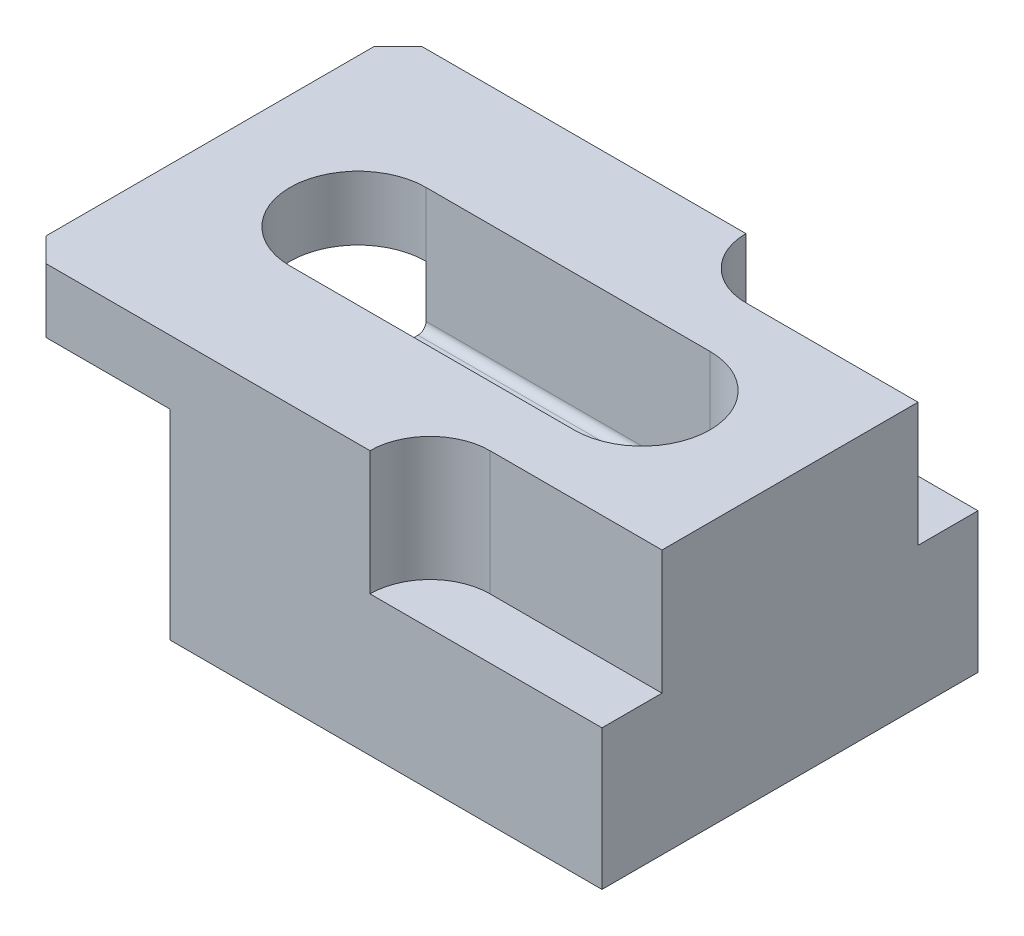
ISO-10303-21;
HEADER;
FILE_DESCRIPTION(('STEP AP214'),'2;1');
FILE_NAME('part.step','',(''),(''),'','','');
FILE_SCHEMA(('AUTOMOTIVE_DESIGN { 1 0 10303 214 1 1 1 1 }'));
ENDSEC;
DATA;
#1=APPLICATION_CONTEXT('core data for automotive mechanical design processes');
#2=APPLICATION_PROTOCOL_DEFINITION('international standard','automotive_design',2000,#1);
#3=PRODUCT_CONTEXT('',#1,'mechanical');
#4=PRODUCT('Part','Part','',(#3));
#5=PRODUCT_RELATED_PRODUCT_CATEGORY('part','',(#4));
#6=PRODUCT_DEFINITION_FORMATION('','',#4);
#7=PRODUCT_DEFINITION_CONTEXT('part definition',#1,'design');
#8=PRODUCT_DEFINITION('design','',#6,#7);
#9=PRODUCT_DEFINITION_SHAPE('','',#8);
#10=(LENGTH_UNIT() NAMED_UNIT(*) SI_UNIT(.MILLI.,.METRE.));
#11=(NAMED_UNIT(*) PLANE_ANGLE_UNIT() SI_UNIT($,.RADIAN.));
#12=(NAMED_UNIT(*) SI_UNIT($,.STERADIAN.) SOLID_ANGLE_UNIT());
#13=UNCERTAINTY_MEASURE_WITH_UNIT(LENGTH_MEASURE(1.E-05),#10,'distance_accuracy_value','');
#14=(GEOMETRIC_REPRESENTATION_CONTEXT(3) GLOBAL_UNCERTAINTY_ASSIGNED_CONTEXT((#13)) GLOBAL_UNIT_ASSIGNED_CONTEXT((#10,
#11,#12)) REPRESENTATION_CONTEXT('',''));
#15=CARTESIAN_POINT('',(0.,0.,0.));
#16=DIRECTION('',(0.,0.,1.));
#17=DIRECTION('',(1.,0.,0.));
#18=AXIS2_PLACEMENT_3D('',#15,#16,#17);
#19=CARTESIAN_POINT('',(-17.75,0.,-8.5));
#20=DIRECTION('',(0.,0.,-1.));
#21=DIRECTION('',(-1.,0.,0.));
#22=AXIS2_PLACEMENT_3D('',#19,#20,#21);
#23=PLANE('',#22);
#24=DIRECTION('',(0.,1.,0.));
#25=VECTOR('',#24,1.);
#26=CARTESIAN_POINT('',(-17.7499999999999,-25.,-8.5));
#27=LINE('',#26,#25);
#28=CARTESIAN_POINT('',(-17.7499999999999,-6.5,-8.5));
#29=VERTEX_POINT('',#28);
#30=CARTESIAN_POINT('',(-17.7499999999999,0.,-8.5));
#31=VERTEX_POINT('',#30);
#32=EDGE_CURVE('E261',#29,#31,#27,.T.);
#33=ORIENTED_EDGE('',*,*,#32,.F.);
#34=DIRECTION('',(-1.,0.,0.));
#35=VECTOR('',#34,1.);
#36=CARTESIAN_POINT('',(17.75,-6.5,-8.5));
#37=LINE('',#36,#35);
#38=CARTESIAN_POINT('',(17.75,-6.5,-8.5));
#39=VERTEX_POINT('',#38);
#40=EDGE_CURVE('E68',#29,#39,#37,.F.);
#41=ORIENTED_EDGE('',*,*,#40,.T.);
#42=DIRECTION('',(0.,1.,0.));
#43=VECTOR('',#42,1.);
#44=CARTESIAN_POINT('',(17.75,0.,-8.5));
#45=LINE('',#44,#43);
#46=CARTESIAN_POINT('',(17.75,8.,-8.5));
#47=VERTEX_POINT('',#46);
#48=EDGE_CURVE('E289',#39,#47,#45,.T.);
#49=ORIENTED_EDGE('',*,*,#48,.T.);
#50=DIRECTION('',(-1.,0.,0.));
#51=VECTOR('',#50,1.);
#52=CARTESIAN_POINT('',(-17.75,8.,-8.5));
#53=LINE('',#52,#51);
#54=CARTESIAN_POINT('',(-17.75,8.,-8.5));
#55=VERTEX_POINT('',#54);
#56=EDGE_CURVE('E273',#47,#55,#53,.T.);
#57=ORIENTED_EDGE('',*,*,#56,.T.);
#58=DIRECTION('',(0.,1.,0.));
#59=VECTOR('',#58,1.);
#60=CARTESIAN_POINT('',(-17.75,0.,-8.5));
#61=LINE('',#60,#59);
#62=EDGE_CURVE('E282',#31,#55,#61,.T.);
#63=ORIENTED_EDGE('',*,*,#62,.F.);
#64=EDGE_LOOP('',(#33,#41,#49,#57,#63));
#65=FACE_BOUND('',#64,.T.);
#66=ADVANCED_FACE('F50',(#65),#23,.F.);
#67=CARTESIAN_POINT('',(17.75,0.,0.));
#68=DIRECTION('',(0.,1.,0.));
#69=DIRECTION('',(0.,0.,1.));
#70=AXIS2_PLACEMENT_3D('',#67,#68,#69);
#71=CYLINDRICAL_SURFACE('',#70,8.5);
#72=ORIENTED_EDGE('',*,*,#48,.F.);
#73=CARTESIAN_POINT('',(17.75,-6.5,0.));
#74=DIRECTION('',(0.,-1.,0.));
#75=DIRECTION('',(0.,0.,-1.));
#76=AXIS2_PLACEMENT_3D('',#73,#74,#75);
#77=CIRCLE('',#76,8.5);
#78=CARTESIAN_POINT('',(17.75,-6.5,8.5));
#79=VERTEX_POINT('',#78);
#80=EDGE_CURVE('E353',#39,#79,#77,.T.);
#81=ORIENTED_EDGE('',*,*,#80,.T.);
#82=DIRECTION('',(0.,1.,0.));
#83=VECTOR('',#82,1.);
#84=CARTESIAN_POINT('',(17.75,0.,8.5));
#85=LINE('',#84,#83);
#86=CARTESIAN_POINT('',(17.75,8.,8.5));
#87=VERTEX_POINT('',#86);
#88=EDGE_CURVE('E290',#79,#87,#85,.T.);
#89=ORIENTED_EDGE('',*,*,#88,.T.);
#90=CARTESIAN_POINT('',(17.75,8.,0.));
#91=DIRECTION('',(0.,1.,0.));
#92=DIRECTION('',(0.,0.,1.));
#93=AXIS2_PLACEMENT_3D('',#90,#91,#92);
#94=CIRCLE('',#93,8.5);
#95=EDGE_CURVE('E278',#87,#47,#94,.T.);
#96=ORIENTED_EDGE('',*,*,#95,.T.);
#97=EDGE_LOOP('',(#72,#81,#89,#96));
#98=FACE_BOUND('',#97,.T.);
#99=ADVANCED_FACE('F388',(#98),#71,.F.);
#100=CARTESIAN_POINT('',(-17.75,0.,8.5));
#101=DIRECTION('',(0.,0.,1.));
#102=DIRECTION('',(1.,0.,0.));
#103=AXIS2_PLACEMENT_3D('',#100,#101,#102);
#104=PLANE('',#103);
#105=ORIENTED_EDGE('',*,*,#88,.F.);
#106=DIRECTION('',(1.,0.,0.));
#107=VECTOR('',#106,1.);
#108=CARTESIAN_POINT('',(-17.75,-6.5,8.5));
#109=LINE('',#108,#107);
#110=CARTESIAN_POINT('',(-17.7499999999999,-6.5,8.5));
#111=VERTEX_POINT('',#110);
#112=EDGE_CURVE('E352',#79,#111,#109,.F.);
#113=ORIENTED_EDGE('',*,*,#112,.T.);
#114=DIRECTION('',(0.,1.,0.));
#115=VECTOR('',#114,1.);
#116=CARTESIAN_POINT('',(-17.7499999999999,-25.,8.5));
#117=LINE('',#116,#115);
#118=CARTESIAN_POINT('',(-17.7499999999999,0.,8.5));
#119=VERTEX_POINT('',#118);
#120=EDGE_CURVE('E258',#111,#119,#117,.T.);
#121=ORIENTED_EDGE('',*,*,#120,.T.);
#122=DIRECTION('',(0.,1.,0.));
#123=VECTOR('',#122,1.);
#124=CARTESIAN_POINT('',(-17.75,0.,8.5));
#125=LINE('',#124,#123);
#126=CARTESIAN_POINT('',(-17.75,8.,8.5));
#127=VERTEX_POINT('',#126);
#128=EDGE_CURVE('E274',#119,#127,#125,.T.);
#129=ORIENTED_EDGE('',*,*,#128,.T.);
#130=DIRECTION('',(1.,0.,0.));
#131=VECTOR('',#130,1.);
#132=CARTESIAN_POINT('',(-17.75,8.,8.5));
#133=LINE('',#132,#131);
#134=EDGE_CURVE('E280',#127,#87,#133,.T.);
#135=ORIENTED_EDGE('',*,*,#134,.T.);
#136=EDGE_LOOP('',(#105,#113,#121,#129,#135));
#137=FACE_BOUND('',#136,.T.);
#138=ADVANCED_FACE('F387',(#137),#104,.F.);
#139=CARTESIAN_POINT('',(7.24999999999998,-17.,16.));
#140=DIRECTION('',(0.,0.,-1.));
#141=DIRECTION('',(-1.,0.,0.));
#142=AXIS2_PLACEMENT_3D('',#139,#140,#141);
#143=PLANE('',#142);
#144=DIRECTION('',(-1.,0.,0.));
#145=VECTOR('',#144,1.);
#146=CARTESIAN_POINT('',(7.24999999999998,-7.5,16.));
#147=LINE('',#146,#145);
#148=CARTESIAN_POINT('',(36.25,-7.5,16.));
#149=VERTEX_POINT('',#148);
#150=CARTESIAN_POINT('',(14.75,-7.5,16.));
#151=VERTEX_POINT('',#150);
#152=EDGE_CURVE('E227',#149,#151,#147,.T.);
#153=ORIENTED_EDGE('',*,*,#152,.F.);
#154=DIRECTION('',(0.,1.,0.));
#155=VECTOR('',#154,1.);
#156=CARTESIAN_POINT('',(36.25,-17.,16.));
#157=LINE('',#156,#155);
#158=CARTESIAN_POINT('',(36.25,8.,16.));
#159=VERTEX_POINT('',#158);
#160=EDGE_CURVE('E237',#149,#159,#157,.T.);
#161=ORIENTED_EDGE('',*,*,#160,.T.);
#162=DIRECTION('',(-1.,0.,0.));
#163=VECTOR('',#162,1.);
#164=CARTESIAN_POINT('',(7.24999999999998,8.,16.));
#165=LINE('',#164,#163);
#166=CARTESIAN_POINT('',(14.75,8.,16.));
#167=VERTEX_POINT('',#166);
#168=EDGE_CURVE('E232',#159,#167,#165,.T.);
#169=ORIENTED_EDGE('',*,*,#168,.T.);
#170=DIRECTION('',(0.,1.,0.));
#171=VECTOR('',#170,1.);
#172=CARTESIAN_POINT('',(14.75,-17.,16.));
#173=LINE('',#172,#171);
#174=EDGE_CURVE('E333',#167,#151,#173,.F.);
#175=ORIENTED_EDGE('',*,*,#174,.T.);
#176=EDGE_LOOP('',(#153,#161,#169,#175));
#177=FACE_BOUND('',#176,.T.);
#178=ADVANCED_FACE('F408',(#177),#143,.F.);
#179=CARTESIAN_POINT('',(36.25,-17.,-16.));
#180=DIRECTION('',(0.,0.,1.));
#181=DIRECTION('',(1.,0.,0.));
#182=AXIS2_PLACEMENT_3D('',#179,#180,#181);
#183=PLANE('',#182);
#184=DIRECTION('',(1.,0.,0.));
#185=VECTOR('',#184,1.);
#186=CARTESIAN_POINT('',(36.25,-7.5,-16.));
#187=LINE('',#186,#185);
#188=CARTESIAN_POINT('',(14.75,-7.5,-16.));
#189=VERTEX_POINT('',#188);
#190=CARTESIAN_POINT('',(36.25,-7.5,-16.));
#191=VERTEX_POINT('',#190);
#192=EDGE_CURVE('E208',#189,#191,#187,.T.);
#193=ORIENTED_EDGE('',*,*,#192,.F.);
#194=DIRECTION('',(0.,1.,0.));
#195=VECTOR('',#194,1.);
#196=CARTESIAN_POINT('',(14.75,8.,-16.));
#197=LINE('',#196,#195);
#198=CARTESIAN_POINT('',(14.75,8.,-16.));
#199=VERTEX_POINT('',#198);
#200=EDGE_CURVE('E332',#189,#199,#197,.T.);
#201=ORIENTED_EDGE('',*,*,#200,.T.);
#202=DIRECTION('',(1.,0.,0.));
#203=VECTOR('',#202,1.);
#204=CARTESIAN_POINT('',(36.25,8.,-16.));
#205=LINE('',#204,#203);
#206=CARTESIAN_POINT('',(36.25,8.,-16.));
#207=VERTEX_POINT('',#206);
#208=EDGE_CURVE('E236',#199,#207,#205,.T.);
#209=ORIENTED_EDGE('',*,*,#208,.T.);
#210=DIRECTION('',(0.,1.,0.));
#211=VECTOR('',#210,1.);
#212=CARTESIAN_POINT('',(36.25,-17.,-16.));
#213=LINE('',#212,#211);
#214=EDGE_CURVE('E239',#191,#207,#213,.T.);
#215=ORIENTED_EDGE('',*,*,#214,.F.);
#216=EDGE_LOOP('',(#193,#201,#209,#215));
#217=FACE_BOUND('',#216,.T.);
#218=ADVANCED_FACE('F454',(#217),#183,.F.);
#219=CARTESIAN_POINT('',(14.75,-17.,-23.5));
#220=DIRECTION('',(0.,-1.,0.));
#221=DIRECTION('',(0.,0.,-1.));
#222=AXIS2_PLACEMENT_3D('',#219,#220,#221);
#223=CYLINDRICAL_SURFACE('',#222,7.5);
#224=CARTESIAN_POINT('',(14.75,-7.5,-23.5));
#225=DIRECTION('',(0.,-1.,0.));
#226=DIRECTION('',(0.,0.,-1.));
#227=AXIS2_PLACEMENT_3D('',#224,#225,#226);
#228=CIRCLE('',#227,7.5);
#229=CARTESIAN_POINT('',(7.24999999999998,-7.5,-23.5));
#230=VERTEX_POINT('',#229);
#231=EDGE_CURVE('E230',#230,#189,#228,.F.);
#232=ORIENTED_EDGE('',*,*,#231,.F.);
#233=DIRECTION('',(0.,1.,0.));
#234=VECTOR('',#233,1.);
#235=CARTESIAN_POINT('',(7.24999999999998,-17.,-23.5));
#236=LINE('',#235,#234);
#237=CARTESIAN_POINT('',(7.24999999999998,8.,-23.5));
#238=VERTEX_POINT('',#237);
#239=EDGE_CURVE('E219',#230,#238,#236,.T.);
#240=ORIENTED_EDGE('',*,*,#239,.T.);
#241=CARTESIAN_POINT('',(14.75,8.,-23.5));
#242=DIRECTION('',(0.,1.,0.));
#243=DIRECTION('',(0.,0.,1.));
#244=AXIS2_PLACEMENT_3D('',#241,#242,#243);
#245=CIRCLE('',#244,7.5);
#246=EDGE_CURVE('E340',#199,#238,#245,.F.);
#247=ORIENTED_EDGE('',*,*,#246,.F.);
#248=ORIENTED_EDGE('',*,*,#200,.F.);
#249=EDGE_LOOP('',(#232,#240,#247,#248));
#250=FACE_BOUND('',#249,.T.);
#251=ADVANCED_FACE('F448',(#250),#223,.F.);
#252=CARTESIAN_POINT('',(14.75,-17.,23.5));
#253=DIRECTION('',(0.,-1.,0.));
#254=DIRECTION('',(0.,0.,-1.));
#255=AXIS2_PLACEMENT_3D('',#252,#253,#254);
#256=CYLINDRICAL_SURFACE('',#255,7.5);
#257=CARTESIAN_POINT('',(14.75,-7.5,23.5));
#258=DIRECTION('',(0.,-1.,0.));
#259=DIRECTION('',(0.,0.,-1.));
#260=AXIS2_PLACEMENT_3D('',#257,#258,#259);
#261=CIRCLE('',#260,7.5);
#262=CARTESIAN_POINT('',(7.24999999999998,-7.5,23.5));
#263=VERTEX_POINT('',#262);
#264=EDGE_CURVE('E345',#151,#263,#261,.F.);
#265=ORIENTED_EDGE('',*,*,#264,.F.);
#266=ORIENTED_EDGE('',*,*,#174,.F.);
#267=CARTESIAN_POINT('',(14.75,8.,23.5));
#268=DIRECTION('',(0.,1.,0.));
#269=DIRECTION('',(0.,0.,1.));
#270=AXIS2_PLACEMENT_3D('',#267,#268,#269);
#271=CIRCLE('',#270,7.5);
#272=CARTESIAN_POINT('',(7.24999999999998,8.,23.5));
#273=VERTEX_POINT('',#272);
#274=EDGE_CURVE('E338',#273,#167,#271,.F.);
#275=ORIENTED_EDGE('',*,*,#274,.F.);
#276=DIRECTION('',(0.,1.,0.));
#277=VECTOR('',#276,1.);
#278=CARTESIAN_POINT('',(7.24999999999998,-17.,23.5));
#279=LINE('',#278,#277);
#280=EDGE_CURVE('E244',#263,#273,#279,.T.);
#281=ORIENTED_EDGE('',*,*,#280,.F.);
#282=EDGE_LOOP('',(#265,#266,#275,#281));
#283=FACE_BOUND('',#282,.T.);
#284=ADVANCED_FACE('F436',(#283),#256,.F.);
#285=CARTESIAN_POINT('',(36.25,8.,-23.5));
#286=DIRECTION('',(-1.,0.,0.));
#287=DIRECTION('',(0.,0.,1.));
#288=AXIS2_PLACEMENT_3D('',#285,#286,#287);
#289=PLANE('',#288);
#290=DIRECTION('',(0.,0.,-1.));
#291=VECTOR('',#290,1.);
#292=CARTESIAN_POINT('',(36.25,-7.5,-23.5));
#293=LINE('',#292,#291);
#294=CARTESIAN_POINT('',(36.25,-7.5,-23.5));
#295=VERTEX_POINT('',#294);
#296=EDGE_CURVE('E191',#191,#295,#293,.T.);
#297=ORIENTED_EDGE('',*,*,#296,.F.);
#298=ORIENTED_EDGE('',*,*,#214,.T.);
#299=DIRECTION('',(0.,0.,-1.));
#300=VECTOR('',#299,1.);
#301=CARTESIAN_POINT('',(36.25,8.,-23.5));
#302=LINE('',#301,#300);
#303=EDGE_CURVE('E295',#159,#207,#302,.T.);
#304=ORIENTED_EDGE('',*,*,#303,.F.);
#305=ORIENTED_EDGE('',*,*,#160,.F.);
#306=CARTESIAN_POINT('',(36.25,-7.5,23.5));
#307=VERTEX_POINT('',#306);
#308=EDGE_CURVE('E212',#307,#149,#293,.T.);
#309=ORIENTED_EDGE('',*,*,#308,.F.);
#310=DIRECTION('',(0.,-1.,0.));
#311=VECTOR('',#310,1.);
#312=CARTESIAN_POINT('',(36.25,8.,23.5));
#313=LINE('',#312,#311);
#314=CARTESIAN_POINT('',(36.25,-25.,23.5));
#315=VERTEX_POINT('',#314);
#316=EDGE_CURVE('E202',#307,#315,#313,.T.);
#317=ORIENTED_EDGE('',*,*,#316,.T.);
#318=DIRECTION('',(0.,0.,-1.));
#319=VECTOR('',#318,1.);
#320=CARTESIAN_POINT('',(36.25,-25.,-23.5));
#321=LINE('',#320,#319);
#322=CARTESIAN_POINT('',(36.25,-25.,-23.5));
#323=VERTEX_POINT('',#322);
#324=EDGE_CURVE('E199',#315,#323,#321,.T.);
#325=ORIENTED_EDGE('',*,*,#324,.T.);
#326=DIRECTION('',(0.,-1.,0.));
#327=VECTOR('',#326,1.);
#328=CARTESIAN_POINT('',(36.25,8.,-23.5));
#329=LINE('',#328,#327);
#330=EDGE_CURVE('E192',#295,#323,#329,.T.);
#331=ORIENTED_EDGE('',*,*,#330,.F.);
#332=EDGE_LOOP('',(#297,#298,#304,#305,#309,#317,#325,#331));
#333=FACE_BOUND('',#332,.T.);
#334=ADVANCED_FACE('F194',(#333),#289,.F.);
#335=CARTESIAN_POINT('',(-36.25,8.,-23.5));
#336=DIRECTION('',(0.,0.,1.));
#337=DIRECTION('',(1.,0.,0.));
#338=AXIS2_PLACEMENT_3D('',#335,#336,#337);
#339=PLANE('',#338);
#340=DIRECTION('',(0.,1.,0.));
#341=VECTOR('',#340,1.);
#342=CARTESIAN_POINT('',(-17.7499999999999,-25.,-23.5));
#343=LINE('',#342,#341);
#344=CARTESIAN_POINT('',(-17.7499999999999,-25.,-23.5));
#345=VERTEX_POINT('',#344);
#346=CARTESIAN_POINT('',(-17.7499999999999,0.,-23.5));
#347=VERTEX_POINT('',#346);
#348=EDGE_CURVE('E257',#345,#347,#343,.T.);
#349=ORIENTED_EDGE('',*,*,#348,.T.);
#350=DIRECTION('',(-1.,0.,0.));
#351=VECTOR('',#350,1.);
#352=CARTESIAN_POINT('',(-36.25,0.,-23.5));
#353=LINE('',#352,#351);
#354=CARTESIAN_POINT('',(-33.25,0.,-23.5));
#355=VERTEX_POINT('',#354);
#356=EDGE_CURVE('E287',#347,#355,#353,.T.);
#357=ORIENTED_EDGE('',*,*,#356,.T.);
#358=DIRECTION('',(0.,1.,0.));
#359=VECTOR('',#358,1.);
#360=CARTESIAN_POINT('',(-33.25,8.,-23.5));
#361=LINE('',#360,#359);
#362=CARTESIAN_POINT('',(-33.25,8.,-23.5));
#363=VERTEX_POINT('',#362);
#364=EDGE_CURVE('E325',#355,#363,#361,.T.);
#365=ORIENTED_EDGE('',*,*,#364,.T.);
#366=DIRECTION('',(-1.,0.,0.));
#367=VECTOR('',#366,1.);
#368=CARTESIAN_POINT('',(-36.25,8.,-23.5));
#369=LINE('',#368,#367);
#370=EDGE_CURVE('E300',#238,#363,#369,.T.);
#371=ORIENTED_EDGE('',*,*,#370,.F.);
#372=ORIENTED_EDGE('',*,*,#239,.F.);
#373=DIRECTION('',(-1.,0.,0.));
#374=VECTOR('',#373,1.);
#375=CARTESIAN_POINT('',(36.25,-7.5,-23.5));
#376=LINE('',#375,#374);
#377=EDGE_CURVE('E209',#295,#230,#376,.T.);
#378=ORIENTED_EDGE('',*,*,#377,.F.);
#379=ORIENTED_EDGE('',*,*,#330,.T.);
#380=DIRECTION('',(-1.,0.,0.));
#381=VECTOR('',#380,1.);
#382=CARTESIAN_POINT('',(36.25,-25.,-23.5));
#383=LINE('',#382,#381);
#384=EDGE_CURVE('E248',#323,#345,#383,.T.);
#385=ORIENTED_EDGE('',*,*,#384,.T.);
#386=EDGE_LOOP('',(#349,#357,#365,#371,#372,#378,#379,#385));
#387=FACE_BOUND('',#386,.T.);
#388=ADVANCED_FACE('F211',(#387),#339,.F.);
#389=CARTESIAN_POINT('',(-36.25,8.,-23.5));
#390=DIRECTION('',(1.,0.,0.));
#391=DIRECTION('',(0.,0.,-1.));
#392=AXIS2_PLACEMENT_3D('',#389,#390,#391);
#393=PLANE('',#392);
#394=DIRECTION('',(0.,0.,1.));
#395=VECTOR('',#394,1.);
#396=CARTESIAN_POINT('',(-36.25,8.,-23.5));
#397=LINE('',#396,#395);
#398=CARTESIAN_POINT('',(-36.25,8.,-20.5));
#399=VERTEX_POINT('',#398);
#400=CARTESIAN_POINT('',(-36.25,8.,20.5));
#401=VERTEX_POINT('',#400);
#402=EDGE_CURVE('E297',#399,#401,#397,.T.);
#403=ORIENTED_EDGE('',*,*,#402,.F.);
#404=DIRECTION('',(0.,-1.,0.));
#405=VECTOR('',#404,1.);
#406=CARTESIAN_POINT('',(-36.25,8.,-20.5));
#407=LINE('',#406,#405);
#408=CARTESIAN_POINT('',(-36.25,0.,-20.5));
#409=VERTEX_POINT('',#408);
#410=EDGE_CURVE('E313',#399,#409,#407,.T.);
#411=ORIENTED_EDGE('',*,*,#410,.T.);
#412=DIRECTION('',(0.,0.,1.));
#413=VECTOR('',#412,1.);
#414=CARTESIAN_POINT('',(-36.25,0.,-23.5));
#415=LINE('',#414,#413);
#416=CARTESIAN_POINT('',(-36.25,0.,20.5));
#417=VERTEX_POINT('',#416);
#418=EDGE_CURVE('E310',#409,#417,#415,.T.);
#419=ORIENTED_EDGE('',*,*,#418,.T.);
#420=DIRECTION('',(0.,1.,0.));
#421=VECTOR('',#420,1.);
#422=CARTESIAN_POINT('',(-36.25,8.,20.5));
#423=LINE('',#422,#421);
#424=EDGE_CURVE('E201',#417,#401,#423,.T.);
#425=ORIENTED_EDGE('',*,*,#424,.T.);
#426=EDGE_LOOP('',(#403,#411,#419,#425));
#427=FACE_BOUND('',#426,.T.);
#428=ADVANCED_FACE('F430',(#427),#393,.F.);
#429=CARTESIAN_POINT('',(-36.25,8.,23.5));
#430=DIRECTION('',(0.,0.,-1.));
#431=DIRECTION('',(-1.,0.,0.));
#432=AXIS2_PLACEMENT_3D('',#429,#430,#431);
#433=PLANE('',#432);
#434=DIRECTION('',(1.,0.,0.));
#435=VECTOR('',#434,1.);
#436=CARTESIAN_POINT('',(-36.25,0.,23.5));
#437=LINE('',#436,#435);
#438=CARTESIAN_POINT('',(-33.25,0.,23.5));
#439=VERTEX_POINT('',#438);
#440=CARTESIAN_POINT('',(-17.7499999999999,0.,23.5));
#441=VERTEX_POINT('',#440);
#442=EDGE_CURVE('E296',#439,#441,#437,.T.);
#443=ORIENTED_EDGE('',*,*,#442,.T.);
#444=DIRECTION('',(0.,1.,0.));
#445=VECTOR('',#444,1.);
#446=CARTESIAN_POINT('',(-17.7499999999999,-25.,23.5));
#447=LINE('',#446,#445);
#448=CARTESIAN_POINT('',(-17.7499999999999,-25.,23.5));
#449=VERTEX_POINT('',#448);
#450=EDGE_CURVE('E260',#449,#441,#447,.T.);
#451=ORIENTED_EDGE('',*,*,#450,.F.);
#452=DIRECTION('',(1.,0.,0.));
#453=VECTOR('',#452,1.);
#454=CARTESIAN_POINT('',(36.25,-25.,23.5));
#455=LINE('',#454,#453);
#456=EDGE_CURVE('E254',#449,#315,#455,.T.);
#457=ORIENTED_EDGE('',*,*,#456,.T.);
#458=ORIENTED_EDGE('',*,*,#316,.F.);
#459=DIRECTION('',(1.,0.,0.));
#460=VECTOR('',#459,1.);
#461=CARTESIAN_POINT('',(36.25,-7.5,23.5));
#462=LINE('',#461,#460);
#463=EDGE_CURVE('E221',#263,#307,#462,.T.);
#464=ORIENTED_EDGE('',*,*,#463,.F.);
#465=ORIENTED_EDGE('',*,*,#280,.T.);
#466=DIRECTION('',(1.,0.,0.));
#467=VECTOR('',#466,1.);
#468=CARTESIAN_POINT('',(-36.25,8.,23.5));
#469=LINE('',#468,#467);
#470=CARTESIAN_POINT('',(-33.25,8.,23.5));
#471=VERTEX_POINT('',#470);
#472=EDGE_CURVE('E303',#471,#273,#469,.T.);
#473=ORIENTED_EDGE('',*,*,#472,.F.);
#474=DIRECTION('',(0.,-1.,0.));
#475=VECTOR('',#474,1.);
#476=CARTESIAN_POINT('',(-33.25,8.,23.5));
#477=LINE('',#476,#475);
#478=EDGE_CURVE('E328',#471,#439,#477,.T.);
#479=ORIENTED_EDGE('',*,*,#478,.T.);
#480=EDGE_LOOP('',(#443,#451,#457,#458,#464,#465,#473,#479));
#481=FACE_BOUND('',#480,.T.);
#482=ADVANCED_FACE('F420',(#481),#433,.F.);
#483=CARTESIAN_POINT('',(0.,8.,0.));
#484=DIRECTION('',(0.,1.,0.));
#485=DIRECTION('',(0.,0.,1.));
#486=AXIS2_PLACEMENT_3D('',#483,#484,#485);
#487=PLANE('',#486);
#488=ORIENTED_EDGE('',*,*,#208,.F.);
#489=ORIENTED_EDGE('',*,*,#246,.T.);
#490=ORIENTED_EDGE('',*,*,#370,.T.);
#491=DIRECTION('',(0.707106781186548,0.,-0.707106781186547));
#492=VECTOR('',#491,1.);
#493=CARTESIAN_POINT('',(-28.375,8.,-28.375));
#494=LINE('',#493,#492);
#495=EDGE_CURVE('E326',#363,#399,#494,.F.);
#496=ORIENTED_EDGE('',*,*,#495,.T.);
#497=ORIENTED_EDGE('',*,*,#402,.T.);
#498=DIRECTION('',(-0.707106781186547,0.,-0.707106781186548));
#499=VECTOR('',#498,1.);
#500=CARTESIAN_POINT('',(-28.375,8.,28.375));
#501=LINE('',#500,#499);
#502=EDGE_CURVE('E323',#401,#471,#501,.F.);
#503=ORIENTED_EDGE('',*,*,#502,.T.);
#504=ORIENTED_EDGE('',*,*,#472,.T.);
#505=ORIENTED_EDGE('',*,*,#274,.T.);
#506=ORIENTED_EDGE('',*,*,#168,.F.);
#507=ORIENTED_EDGE('',*,*,#303,.T.);
#508=EDGE_LOOP('',(#488,#489,#490,#496,#497,#503,#504,#505,#506,#507));
#509=FACE_BOUND('',#508,.T.);
#510=ORIENTED_EDGE('',*,*,#134,.F.);
#511=CARTESIAN_POINT('',(-17.75,8.,0.));
#512=DIRECTION('',(0.,1.,0.));
#513=DIRECTION('',(0.,0.,1.));
#514=AXIS2_PLACEMENT_3D('',#511,#512,#513);
#515=CIRCLE('',#514,8.5);
#516=EDGE_CURVE('E270',#55,#127,#515,.T.);
#517=ORIENTED_EDGE('',*,*,#516,.F.);
#518=ORIENTED_EDGE('',*,*,#56,.F.);
#519=ORIENTED_EDGE('',*,*,#95,.F.);
#520=EDGE_LOOP('',(#510,#517,#518,#519));
#521=FACE_BOUND('',#520,.T.);
#522=ADVANCED_FACE('F417',(#509,#521),#487,.T.);
#523=CARTESIAN_POINT('',(0.,0.,0.));
#524=DIRECTION('',(0.,1.,0.));
#525=DIRECTION('',(0.,0.,1.));
#526=AXIS2_PLACEMENT_3D('',#523,#524,#525);
#527=PLANE('',#526);
#528=CARTESIAN_POINT('',(-17.75,0.,0.));
#529=DIRECTION('',(0.,1.,0.));
#530=DIRECTION('',(0.,0.,1.));
#531=AXIS2_PLACEMENT_3D('',#528,#529,#530);
#532=CIRCLE('',#531,8.5);
#533=EDGE_CURVE('E272',#31,#119,#532,.T.);
#534=ORIENTED_EDGE('',*,*,#533,.T.);
#535=DIRECTION('',(0.,0.,1.));
#536=VECTOR('',#535,1.);
#537=CARTESIAN_POINT('',(-17.7499999999999,0.,0.));
#538=LINE('',#537,#536);
#539=EDGE_CURVE('E256',#119,#441,#538,.T.);
#540=ORIENTED_EDGE('',*,*,#539,.T.);
#541=ORIENTED_EDGE('',*,*,#442,.F.);
#542=DIRECTION('',(0.707106781186547,0.,0.707106781186548));
#543=VECTOR('',#542,1.);
#544=CARTESIAN_POINT('',(-33.25,0.,23.5));
#545=LINE('',#544,#543);
#546=EDGE_CURVE('E320',#439,#417,#545,.F.);
#547=ORIENTED_EDGE('',*,*,#546,.T.);
#548=ORIENTED_EDGE('',*,*,#418,.F.);
#549=DIRECTION('',(-0.707106781186548,0.,0.707106781186547));
#550=VECTOR('',#549,1.);
#551=CARTESIAN_POINT('',(-36.25,0.,-20.5));
#552=LINE('',#551,#550);
#553=EDGE_CURVE('E316',#409,#355,#552,.F.);
#554=ORIENTED_EDGE('',*,*,#553,.T.);
#555=ORIENTED_EDGE('',*,*,#356,.F.);
#556=DIRECTION('',(0.,0.,1.));
#557=VECTOR('',#556,1.);
#558=CARTESIAN_POINT('',(-17.7499999999999,0.,0.));
#559=LINE('',#558,#557);
#560=EDGE_CURVE('E267',#347,#31,#559,.T.);
#561=ORIENTED_EDGE('',*,*,#560,.T.);
#562=EDGE_LOOP('',(#534,#540,#541,#547,#548,#554,#555,#561));
#563=FACE_BOUND('',#562,.T.);
#564=ADVANCED_FACE('F412',(#563),#527,.F.);
#565=CARTESIAN_POINT('',(-17.75,0.,0.));
#566=DIRECTION('',(0.,1.,0.));
#567=DIRECTION('',(0.,0.,1.));
#568=AXIS2_PLACEMENT_3D('',#565,#566,#567);
#569=CYLINDRICAL_SURFACE('',#568,8.5);
#570=ORIENTED_EDGE('',*,*,#516,.T.);
#571=ORIENTED_EDGE('',*,*,#128,.F.);
#572=ORIENTED_EDGE('',*,*,#533,.F.);
#573=ORIENTED_EDGE('',*,*,#62,.T.);
#574=EDGE_LOOP('',(#570,#571,#572,#573));
#575=FACE_BOUND('',#574,.T.);
#576=ADVANCED_FACE('F414',(#575),#569,.F.);
#577=CARTESIAN_POINT('',(-36.25,8.,-20.5));
#578=DIRECTION('',(0.707106781186547,0.,0.707106781186548));
#579=DIRECTION('',(0.,-1.,0.));
#580=AXIS2_PLACEMENT_3D('',#577,#578,#579);
#581=PLANE('',#580);
#582=ORIENTED_EDGE('',*,*,#495,.F.);
#583=ORIENTED_EDGE('',*,*,#364,.F.);
#584=ORIENTED_EDGE('',*,*,#553,.F.);
#585=ORIENTED_EDGE('',*,*,#410,.F.);
#586=EDGE_LOOP('',(#582,#583,#584,#585));
#587=FACE_BOUND('',#586,.T.);
#588=ADVANCED_FACE('F413',(#587),#581,.F.);
#589=CARTESIAN_POINT('',(-33.25,8.,23.5));
#590=DIRECTION('',(0.707106781186548,0.,-0.707106781186547));
#591=DIRECTION('',(0.,-1.,0.));
#592=AXIS2_PLACEMENT_3D('',#589,#590,#591);
#593=PLANE('',#592);
#594=ORIENTED_EDGE('',*,*,#502,.F.);
#595=ORIENTED_EDGE('',*,*,#424,.F.);
#596=ORIENTED_EDGE('',*,*,#546,.F.);
#597=ORIENTED_EDGE('',*,*,#478,.F.);
#598=EDGE_LOOP('',(#594,#595,#596,#597));
#599=FACE_BOUND('',#598,.T.);
#600=ADVANCED_FACE('F442',(#599),#593,.F.);
#601=CARTESIAN_POINT('',(-17.7499999999999,-25.,-23.5));
#602=DIRECTION('',(-1.,0.,0.));
#603=DIRECTION('',(0.,0.,1.));
#604=AXIS2_PLACEMENT_3D('',#601,#602,#603);
#605=PLANE('',#604);
#606=DIRECTION('',(0.,0.,1.));
#607=VECTOR('',#606,1.);
#608=CARTESIAN_POINT('',(-17.75,-7.5,-23.5));
#609=LINE('',#608,#607);
#610=CARTESIAN_POINT('',(-17.75,-7.5,-7.5));
#611=VERTEX_POINT('',#610);
#612=CARTESIAN_POINT('',(-17.75,-7.5,7.5));
#613=VERTEX_POINT('',#612);
#614=EDGE_CURVE('E220',#611,#613,#609,.T.);
#615=ORIENTED_EDGE('',*,*,#614,.F.);
#616=CARTESIAN_POINT('',(-17.7499999999999,-6.5,-7.5));
#617=DIRECTION('',(-1.,0.,0.));
#618=DIRECTION('',(0.,0.,1.));
#619=AXIS2_PLACEMENT_3D('',#616,#617,#618);
#620=CIRCLE('',#619,1.);
#621=EDGE_CURVE('E11',#611,#29,#620,.F.);
#622=ORIENTED_EDGE('',*,*,#621,.T.);
#623=ORIENTED_EDGE('',*,*,#32,.T.);
#624=ORIENTED_EDGE('',*,*,#560,.F.);
#625=ORIENTED_EDGE('',*,*,#348,.F.);
#626=DIRECTION('',(0.,0.,1.));
#627=VECTOR('',#626,1.);
#628=CARTESIAN_POINT('',(-17.7499999999999,-25.,-23.5));
#629=LINE('',#628,#627);
#630=EDGE_CURVE('E252',#345,#449,#629,.T.);
#631=ORIENTED_EDGE('',*,*,#630,.T.);
#632=ORIENTED_EDGE('',*,*,#450,.T.);
#633=ORIENTED_EDGE('',*,*,#539,.F.);
#634=ORIENTED_EDGE('',*,*,#120,.F.);
#635=CARTESIAN_POINT('',(-17.7499999999999,-6.5,7.5));
#636=DIRECTION('',(-1.,0.,0.));
#637=DIRECTION('',(0.,0.,1.));
#638=AXIS2_PLACEMENT_3D('',#635,#636,#637);
#639=CIRCLE('',#638,1.);
#640=EDGE_CURVE('E57',#111,#613,#639,.F.);
#641=ORIENTED_EDGE('',*,*,#640,.T.);
#642=EDGE_LOOP('',(#615,#622,#623,#624,#625,#631,#632,#633,#634,#641));
#643=FACE_BOUND('',#642,.T.);
#644=ADVANCED_FACE('F382',(#643),#605,.T.);
#645=CARTESIAN_POINT('',(17.75,-25.,0.));
#646=DIRECTION('',(0.,1.,0.));
#647=DIRECTION('',(0.,0.,1.));
#648=AXIS2_PLACEMENT_3D('',#645,#646,#647);
#649=PLANE('',#648);
#650=CARTESIAN_POINT('',(17.75,-25.,0.));
#651=DIRECTION('',(0.,1.,0.));
#652=DIRECTION('',(0.,0.,1.));
#653=AXIS2_PLACEMENT_3D('',#650,#651,#652);
#654=CIRCLE('',#653,4.);
#655=CARTESIAN_POINT('',(17.75,-25.,4.));
#656=VERTEX_POINT('',#655);
#657=EDGE_CURVE('E235',#656,#656,#654,.T.);
#658=ORIENTED_EDGE('',*,*,#657,.T.);
#659=EDGE_LOOP('',(#658));
#660=FACE_BOUND('',#659,.T.);
#661=ORIENTED_EDGE('',*,*,#324,.F.);
#662=ORIENTED_EDGE('',*,*,#456,.F.);
#663=ORIENTED_EDGE('',*,*,#630,.F.);
#664=ORIENTED_EDGE('',*,*,#384,.F.);
#665=EDGE_LOOP('',(#661,#662,#663,#664));
#666=FACE_BOUND('',#665,.T.);
#667=ADVANCED_FACE('F505',(#660,#666),#649,.F.);
#668=CARTESIAN_POINT('',(17.75,-42.,0.));
#669=DIRECTION('',(0.,1.,0.));
#670=DIRECTION('',(0.,0.,1.));
#671=AXIS2_PLACEMENT_3D('',#668,#669,#670);
#672=CYLINDRICAL_SURFACE('',#671,4.);
#673=ORIENTED_EDGE('',*,*,#657,.F.);
#674=EDGE_LOOP('',(#673));
#675=FACE_BOUND('',#674,.T.);
#676=CARTESIAN_POINT('',(17.75,-7.5,0.));
#677=DIRECTION('',(0.,1.,0.));
#678=DIRECTION('',(0.,0.,1.));
#679=AXIS2_PLACEMENT_3D('',#676,#677,#678);
#680=CIRCLE('',#679,4.);
#681=CARTESIAN_POINT('',(17.75,-7.5,4.));
#682=VERTEX_POINT('',#681);
#683=EDGE_CURVE('E215',#682,#682,#680,.T.);
#684=ORIENTED_EDGE('',*,*,#683,.T.);
#685=EDGE_LOOP('',(#684));
#686=FACE_BOUND('',#685,.T.);
#687=ADVANCED_FACE('F369',(#675,#686),#672,.F.);
#688=CARTESIAN_POINT('',(0.,-7.5,0.));
#689=DIRECTION('',(0.,-1.,0.));
#690=DIRECTION('',(0.,0.,-1.));
#691=AXIS2_PLACEMENT_3D('',#688,#689,#690);
#692=PLANE('',#691);
#693=ORIENTED_EDGE('',*,*,#683,.F.);
#694=EDGE_LOOP('',(#693));
#695=FACE_BOUND('',#694,.T.);
#696=ORIENTED_EDGE('',*,*,#614,.T.);
#697=DIRECTION('',(1.,0.,0.));
#698=VECTOR('',#697,1.);
#699=CARTESIAN_POINT('',(17.75,-7.5,7.5));
#700=LINE('',#699,#698);
#701=CARTESIAN_POINT('',(17.75,-7.5,7.5));
#702=VERTEX_POINT('',#701);
#703=EDGE_CURVE('E348',#613,#702,#700,.T.);
#704=ORIENTED_EDGE('',*,*,#703,.T.);
#705=CARTESIAN_POINT('',(17.75,-7.5,0.));
#706=DIRECTION('',(0.,-1.,0.));
#707=DIRECTION('',(0.,0.,-1.));
#708=AXIS2_PLACEMENT_3D('',#705,#706,#707);
#709=CIRCLE('',#708,7.5);
#710=CARTESIAN_POINT('',(17.75,-7.5,-7.5));
#711=VERTEX_POINT('',#710);
#712=EDGE_CURVE('E346',#702,#711,#709,.F.);
#713=ORIENTED_EDGE('',*,*,#712,.T.);
#714=DIRECTION('',(-1.,0.,0.));
#715=VECTOR('',#714,1.);
#716=CARTESIAN_POINT('',(-17.75,-7.5,-7.5));
#717=LINE('',#716,#715);
#718=EDGE_CURVE('E343',#711,#611,#717,.T.);
#719=ORIENTED_EDGE('',*,*,#718,.T.);
#720=EDGE_LOOP('',(#696,#704,#713,#719));
#721=FACE_BOUND('',#720,.T.);
#722=ADVANCED_FACE('F375',(#695,#721),#692,.F.);
#723=ORIENTED_EDGE('',*,*,#308,.T.);
#724=ORIENTED_EDGE('',*,*,#152,.T.);
#725=ORIENTED_EDGE('',*,*,#264,.T.);
#726=ORIENTED_EDGE('',*,*,#463,.T.);
#727=EDGE_LOOP('',(#723,#724,#725,#726));
#728=FACE_BOUND('',#727,.T.);
#729=ADVANCED_FACE('F374',(#728),#692,.F.);
#730=ORIENTED_EDGE('',*,*,#231,.T.);
#731=ORIENTED_EDGE('',*,*,#192,.T.);
#732=ORIENTED_EDGE('',*,*,#296,.T.);
#733=ORIENTED_EDGE('',*,*,#377,.T.);
#734=EDGE_LOOP('',(#730,#731,#732,#733));
#735=FACE_BOUND('',#734,.T.);
#736=ADVANCED_FACE('F206',(#735),#692,.F.);
#737=CARTESIAN_POINT('',(0.,-6.5,-7.5));
#738=DIRECTION('',(1.,0.,0.));
#739=DIRECTION('',(0.,0.,-1.));
#740=AXIS2_PLACEMENT_3D('',#737,#738,#739);
#741=CYLINDRICAL_SURFACE('',#740,1.);
#742=ORIENTED_EDGE('',*,*,#621,.F.);
#743=ORIENTED_EDGE('',*,*,#718,.F.);
#744=CARTESIAN_POINT('',(17.75,-6.5,-7.5));
#745=DIRECTION('',(-1.,0.,0.));
#746=DIRECTION('',(0.,0.,1.));
#747=AXIS2_PLACEMENT_3D('',#744,#745,#746);
#748=CIRCLE('',#747,1.);
#749=EDGE_CURVE('E51',#39,#711,#748,.T.);
#750=ORIENTED_EDGE('',*,*,#749,.F.);
#751=ORIENTED_EDGE('',*,*,#40,.F.);
#752=EDGE_LOOP('',(#742,#743,#750,#751));
#753=FACE_BOUND('',#752,.T.);
#754=ADVANCED_FACE('F47',(#753),#741,.F.);
#755=CARTESIAN_POINT('',(17.75,-6.5,0.));
#756=DIRECTION('',(0.,-1.,0.));
#757=DIRECTION('',(0.,0.,-1.));
#758=AXIS2_PLACEMENT_3D('',#755,#756,#757);
#759=TOROIDAL_SURFACE('',#758,7.5,1.);
#760=ORIENTED_EDGE('',*,*,#749,.T.);
#761=ORIENTED_EDGE('',*,*,#712,.F.);
#762=CARTESIAN_POINT('',(17.75,-6.5,7.5));
#763=DIRECTION('',(1.,0.,0.));
#764=DIRECTION('',(0.,0.,-1.));
#765=AXIS2_PLACEMENT_3D('',#762,#763,#764);
#766=CIRCLE('',#765,1.);
#767=EDGE_CURVE('E357',#79,#702,#766,.T.);
#768=ORIENTED_EDGE('',*,*,#767,.F.);
#769=ORIENTED_EDGE('',*,*,#80,.F.);
#770=EDGE_LOOP('',(#760,#761,#768,#769));
#771=FACE_BOUND('',#770,.T.);
#772=ADVANCED_FACE('F391',(#771),#759,.F.);
#773=CARTESIAN_POINT('',(0.,-6.5,7.5));
#774=DIRECTION('',(-1.,0.,0.));
#775=DIRECTION('',(0.,0.,1.));
#776=AXIS2_PLACEMENT_3D('',#773,#774,#775);
#777=CYLINDRICAL_SURFACE('',#776,1.);
#778=ORIENTED_EDGE('',*,*,#640,.F.);
#779=ORIENTED_EDGE('',*,*,#112,.F.);
#780=ORIENTED_EDGE('',*,*,#767,.T.);
#781=ORIENTED_EDGE('',*,*,#703,.F.);
#782=EDGE_LOOP('',(#778,#779,#780,#781));
#783=FACE_BOUND('',#782,.T.);
#784=ADVANCED_FACE('F378',(#783),#777,.F.);
#785=CLOSED_SHELL('',(#66,#99,#138,#178,#218,#251,#284,#334,#388,#428,#482,#522,#564,#576,#588,
#600,#644,#667,#687,#722,#729,#736,#754,#772,#784));
#786=MANIFOLD_SOLID_BREP('B2',#785);
#787=ADVANCED_BREP_SHAPE_REPRESENTATION('',(#18,#786),#14);
#788=SHAPE_DEFINITION_REPRESENTATION(#9,#787);
ENDSEC;
END-ISO-10303-21;
